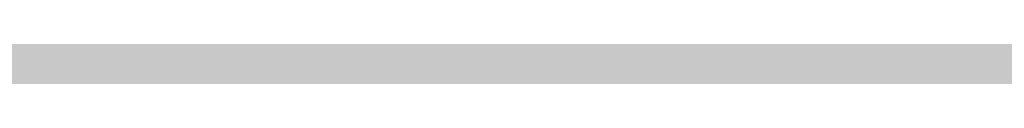
# Model space of a CAD drawing. Units: millimetres. Extents: x 0 to 2267, y 0 to 1823.
# Tile 105 of 256: x 1600.369 to 1605.705, y 1232.061 to 1232.196. Entities that reach past the tile are written whole.
import ezdxf

# ---------------------------------------------------------------- set-up
doc = ezdxf.new("R2010")
doc.units = ezdxf.units.MM
doc.header["$MEASUREMENT"] = 0
doc.layers.add('M-DIMS', color=2, linetype='Continuous', lineweight=25)
doc.layers.add('M-HATC', color=252, linetype='Continuous', lineweight=18)
doc.styles.get("Standard").update_dxf_attribs({"font": 'arial.ttf'})
doc.dimstyles.get("Standard").update_dxf_attribs({"dimtxt": 7, "dimasz": 4, "dimexe": 0.18, "dimexo": 0.0625, "dimgap": 0.09, "dimtad": 0, "dimdec": 0, "dimzin": 0, "dimdsep": 46, "dimtxsty": 'Standard', "dimcen": 0.09, "dimadec": 0, "dimazin": 0, "dimtfac": 1, "dimtdec": 0, "dimtofl": 0, "dimtmove": 0, "dimatfit": 3, "dimfxl": 1, "dimtolj": 1, "dimtzin": 0, "dimarcsym": 0})

# ---------------------------------------------------------------- blocks, each defined once
blk = doc.blocks.new('*D19')
at = {"layer": 'Defpoints', "color": 0, "transparency": 16777216}
for p in [(1605.3399, 1483.3044), (1445.5291, 1333.8851)]:
    blk.add_point(p, dxfattribs=at)
at = {"layer": 'M-DIMS', "color": 0, "lineweight": -2, "transparency": 16777216}
for p, q in [((1605.3399, 1483.2144), (1605.3399, 1483.3944)), ((1605.2499, 1483.3044), (1605.4299, 1483.3044)), ((1366.3244, 1259.8306), (1442.6072, 1331.1532))]:
    blk.add_line(p, q, dxfattribs=at)
at = {"layer": 'M-DIMS', "color": 0, "transparency": 16777216}
blk.add_solid([(1442.1519, 1331.6402), (1443.0625, 1330.6663), (1445.5291, 1333.8851)], dxfattribs=at)
at = {"layer": 'M-DIMS', "color": 0, "transparency": 16777216, "insert": (1349.6425, 1244.2335), "char_height": 7, "attachment_point": 5, "rotation": 43.0753}
blk.add_mtext('\\A1;2X R218.8', dxfattribs=at)

msp = doc.modelspace()

# ---------------------------------------------------------------- hatches: boundary and pattern name
at = {"layer": 'M-HATC'}
h = msp.add_hatch(color=256, dxfattribs=at)
h.dxf.hatch_style = 1
h.paths.add_polyline_path([(2055.771, 1603.062), (1381.0868, 1603.062), (1381.0868, 1598.062), (2055.771, 1598.062)])
h.paths.add_polyline_path([(2055.771, 1598.062), (1381.0868, 1598.062), (1381.0868, 1593.062), (2055.771, 1593.062)])
h.paths.add_polyline_path([(2051.3074, 1536.7609), (1385.5504, 1536.7609), (1385.5504, 1526.7609), (1387.5504, 1526.7609), (1388.5366, 1525.0528), (1385.3319, 1521.2335), (1385.3319, 1521.2226), (2050.2542, 1522.7491), (2048.3212, 1525.0528), (2049.3074, 1526.7609), (2051.3074, 1526.7609)])
edge = h.paths.add_edge_path()
edge.add_arc((1847.5345, 1379.1492), 135, 222.603061, 222.890851, ccw=False)
edge.add_line((1748.1663, 1287.7656), (1683.0921, 1287.7656))
edge.add_arc((1583.7239, 1379.1492), 135, 317.109149, 317.396939, ccw=False)
edge.add_arc((1678.9686, 1290.6707), 5, 222.8909, 317.1091, ccw=False)
edge.add_arc((1774.2133, 1379.1492), 135, 222.603061, 222.890851, ccw=False)
edge.add_line((1674.8451, 1287.7656), (1609.7709, 1287.7656))
edge.add_arc((1510.4027, 1379.1492), 135, 317.109149, 317.396939, ccw=False)
edge.add_arc((1605.6474, 1290.6707), 5, 222.8909, 317.1091, ccw=False)
edge.add_arc((1700.8921, 1379.1492), 135, 222.603061, 222.890851, ccw=False)
edge.add_line((1601.5239, 1287.7656), (1536.4497, 1287.7656))
edge.add_arc((1437.0815, 1379.1492), 135, 317.109149, 317.396939, ccw=False)
edge.add_arc((1532.3262, 1290.6707), 5, 222.8909, 317.1091, ccw=False)
edge.add_arc((1627.5709, 1379.1492), 135, 222.603061, 222.890851, ccw=False)
edge.add_line((1528.2027, 1287.7656), (1505.9289, 1287.7656))
edge.add_spline(control_points=[(1505.9289, 1287.7656), (1504.2622, 1287.7656), (1504.2622, 1282.7656), (1505.9289, 1282.7656)], knot_values=[0, 0, 0, 0, 5, 5, 5, 5], degree=3, periodic=0)
edge.add_line((1505.9289, 1282.7656), (1930.9289, 1282.7656))
edge.add_spline(control_points=[(1930.9289, 1282.7656), (1932.5956, 1282.7656), (1932.5956, 1287.7656), (1930.9289, 1287.7656)], knot_values=[0, 0, 0, 0, 5, 5, 5, 5], degree=3, periodic=0)
edge.add_line((1930.9289, 1287.7656), (1903.0557, 1287.7656))
edge.add_arc((1803.6875, 1379.1492), 135, 317.109149, 317.396939, ccw=False)
edge.add_arc((1898.9322, 1290.6707), 5, 222.8909, 317.1091, ccw=False)
edge.add_arc((1994.1769, 1379.1492), 135, 222.603061, 222.890851, ccw=False)
edge.add_line((1894.8087, 1287.7656), (1829.7345, 1287.7656))
edge.add_arc((1730.3663, 1379.1492), 135, 317.109149, 317.396939, ccw=False)
edge.add_arc((1825.611, 1290.6707), 5, 222.8909, 317.1091, ccw=False)
edge.add_arc((1920.8557, 1379.1492), 135, 222.603061, 222.890851, ccw=False)
edge.add_line((1821.4875, 1287.7656), (1756.4133, 1287.7656))
edge.add_arc((1657.0451, 1379.1492), 135, 317.109149, 317.396939, ccw=False)
edge.add_arc((1752.2898, 1290.6707), 5, 222.8909, 317.1091, ccw=False)
edge = h.paths.add_edge_path()
edge.add_spline(control_points=[(1843.4289, 1227.2475), (1845.0956, 1227.2475), (1845.0956, 1232.2475), (1843.4289, 1232.2475)], knot_values=[0, 0, 0, 0, 5, 5, 5, 5], degree=3, periodic=0)
edge.add_line((1843.4289, 1232.2475), (1593.4289, 1232.2475))
edge.add_spline(control_points=[(1593.4289, 1232.2475), (1591.7622, 1232.2475), (1591.7622, 1227.2475), (1593.4289, 1227.2475)], knot_values=[0, 0, 0, 0, 5, 5, 5, 5], degree=3, periodic=0)
edge.add_line((1593.4289, 1227.2475), (1843.4289, 1227.2475))
h.paths.add_polyline_path([(1905.9289, 1127.4171), (1530.9289, 1127.4171, 0.414214), (1520.9289, 1117.4171), (1530.9289, 1117.4171), (1915.9289, 1117.4171, 0.414214)])
edge = h.paths.add_edge_path()
edge.add_arc((1397.0858, 1498.4078), 12.7299, 90.78215, 190.87871, ccw=False)
edge.add_line((1396.912, 1511.1365), (1428.0097, 1511.3488))
edge.add_line((1428.0097, 1511.3488), (1433.0097, 1511.3488))
edge.add_line((1433.0097, 1511.3488), (1434.439, 1511.3488))
edge.add_arc((1419.474, 1498.0804), 20, 41.561, 74.08211)
edge.add_line((1424.9592, 1517.3135), (1399.9351, 1517.2561))
edge.add_spline(control_points=[(1399.9307, 1517.2561), (1399.884, 1517.2131), (1399.8328, 1517.1689), (1399.7774, 1517.1236)], knot_values=[11.567499, 11.567499, 11.567499, 11.567499, 11.814249, 11.814249, 11.814249, 11.814249], degree=3, periodic=0)
edge.add_spline(control_points=[(1399.6328, 1517.0099), (1399.5831, 1516.9721), (1399.5307, 1516.9338), (1399.4759, 1516.8947)], knot_values=[11.167718, 11.167718, 11.167718, 11.167718, 11.365188, 11.365188, 11.365188, 11.365188], degree=3, periodic=0)
edge.add_spline(control_points=[(1399.3398, 1516.8001), (1399.1514, 1516.6719), (1398.9384, 1516.5377), (1398.704, 1516.3994)], knot_values=[10.376405, 10.376405, 10.376405, 10.376405, 11.00994, 11.00994, 11.00994, 11.00994], degree=3, periodic=0)
edge.add_spline(control_points=[(1398.6572, 1516.3719), (1398.5789, 1516.326), (1398.4983, 1516.2797), (1398.4155, 1516.2331)], knot_values=[10.125175, 10.125175, 10.125175, 10.125175, 10.334406, 10.334406, 10.334406, 10.334406], degree=3, periodic=0)
edge.add_spline(control_points=[(1398.2642, 1516.1487), (1398.196, 1516.1111), (1398.1263, 1516.0732), (1398.0555, 1516.0351)], knot_values=[9.832246, 9.832246, 9.832246, 9.832246, 9.999658, 9.999658, 9.999658, 9.999658], degree=3, periodic=0)
edge.add_spline(control_points=[(1397.9987, 1516.0048), (1397.7312, 1515.8621), (1397.446, 1515.7171), (1397.1466, 1515.5714)], knot_values=[9.161808, 9.161808, 9.161808, 9.161808, 9.787769, 9.787769, 9.787769, 9.787769], degree=3, periodic=0)
edge.add_spline(control_points=[(1397.1466, 1515.5714), (1396.8418, 1515.423), (1396.5222, 1515.274), (1396.1914, 1515.1262)], knot_values=[8.524455, 8.524455, 8.524455, 8.524455, 9.161808, 9.161808, 9.161808, 9.161808], degree=3, periodic=0)
edge.add_spline(control_points=[(1396.0777, 1515.0756), (1395.9854, 1515.0348), (1395.8922, 1514.994), (1395.7983, 1514.9534)], knot_values=[8.275193, 8.275193, 8.275193, 8.275193, 8.451726, 8.451726, 8.451726, 8.451726], degree=3, periodic=0)
edge.add_spline(control_points=[(1395.6018, 1514.8691), (1395.4997, 1514.8257), (1395.3968, 1514.7824), (1395.2932, 1514.7394)], knot_values=[7.962917, 7.962917, 7.962917, 7.962917, 8.152764, 8.152764, 8.152764, 8.152764], degree=3, periodic=0)
edge.add_spline(control_points=[(1395.2116, 1514.7057), (1394.8278, 1514.5475), (1394.4345, 1514.3929), (1394.0364, 1514.2442)], knot_values=[7.21254, 7.21254, 7.21254, 7.21254, 7.913148, 7.913148, 7.913148, 7.913148], degree=3, periodic=0)
edge.add_spline(control_points=[(1394.0364, 1514.2442), (1393.7076, 1514.1214), (1393.3754, 1514.0027), (1393.0427, 1513.8895)], knot_values=[6.633733, 6.633733, 6.633733, 6.633733, 7.21254, 7.21254, 7.21254, 7.21254], degree=3, periodic=0)
edge.add_spline(control_points=[(1392.8214, 1513.815), (1392.7198, 1513.7812), (1392.6181, 1513.7479), (1392.5166, 1513.7152)], knot_values=[6.328796, 6.328796, 6.328796, 6.328796, 6.505493, 6.505493, 6.505493, 6.505493], degree=3, periodic=0)
edge.add_spline(control_points=[(1392.5166, 1513.7152), (1392.3187, 1513.6515), (1392.1212, 1513.59), (1391.9244, 1513.531)], knot_values=[5.984605, 5.984605, 5.984605, 5.984605, 6.328796, 6.328796, 6.328796, 6.328796], degree=3, periodic=0)
edge.add_spline(control_points=[(1391.7915, 1513.4915), (1391.3122, 1513.3501), (1390.8384, 1513.2239), (1390.3784, 1513.1171)], knot_values=[5.066697, 5.066697, 5.066697, 5.066697, 5.907055, 5.907055, 5.907055, 5.907055], degree=3, periodic=0)
edge.add_spline(control_points=[(1390.3784, 1513.1171), (1390.1797, 1513.071), (1389.9836, 1513.0284), (1389.7907, 1512.9899)], knot_values=[4.70367, 4.70367, 4.70367, 4.70367, 5.066695, 5.066695, 5.066695, 5.066695], degree=3, periodic=0)
edge.add_spline(control_points=[(1389.422, 1512.9204), (1389.2459, 1512.8892), (1389.0729, 1512.8617), (1388.9036, 1512.8381)], knot_values=[4.130571, 4.130571, 4.130571, 4.130571, 4.469816, 4.469816, 4.469816, 4.469816], degree=3, periodic=0)
edge.add_spline(control_points=[(1388.9036, 1512.8381), (1388.591, 1512.7946), (1388.2911, 1512.7644), (1388.0071, 1512.7494)], knot_values=[3.504031, 3.504031, 3.504031, 3.504031, 4.130571, 4.130571, 4.130571, 4.130571], degree=3, periodic=0)
edge.add_spline(control_points=[(1387.9356, 1512.7459), (1387.8538, 1512.7423), (1387.7733, 1512.74), (1387.6944, 1512.739)], knot_values=[3.268866, 3.268866, 3.268866, 3.268866, 3.451164, 3.451164, 3.451164, 3.451164], degree=3, periodic=0)
edge.add_spline(control_points=[(1387.3351, 1512.7443), (1387.2076, 1512.7499), (1387.0847, 1512.7597), (1386.967, 1512.7739)], knot_values=[2.670686, 2.670686, 2.670686, 2.670686, 2.984, 2.984, 2.984, 2.984], degree=3, periodic=0)
edge.add_spline(control_points=[(1386.8327, 1512.7922), (1386.8209, 1512.7941), (1386.8092, 1512.7959), (1386.7975, 1512.7979)], knot_values=[2.516981, 2.516981, 2.516981, 2.516981, 2.549528, 2.549528, 2.549528, 2.549528], degree=3, periodic=0)
edge.add_spline(control_points=[(1386.4526, 1512.8735), (1386.4257, 1512.881), (1386.3993, 1512.889), (1386.3733, 1512.8972)], knot_values=[2.095869, 2.095869, 2.095869, 2.095869, 2.17941, 2.17941, 2.17941, 2.17941], degree=3, periodic=0)
edge.add_spline(control_points=[(1386.0691, 1513.0189), (1386.0634, 1513.0217), (1386.0577, 1513.0246), (1386.052, 1513.0275)], knot_values=[1.72453, 1.72453, 1.72453, 1.72453, 1.745933, 1.745933, 1.745933, 1.745933], degree=3, periodic=0)
edge.add_arc((1399.474, 1498.0804), 20, 131.82432, 180)
edge.add_arc((1630.3336, 1505.5484), 250.9708, 181.705176, 236.427975)
edge.add_arc((1605.3399, 1483.3044), 218.7822, 238.660829, 243.34961)
edge.add_arc((1647.0911, 1510.3592), 262.8986, 183.129836, 237.853442, ccw=False)
h.paths.add_polyline_path([(1406.5369, 1391.9644, 0.149382), (1491.5506, 1296.4418, -0.129517)], flags=17)
edge = h.paths.add_edge_path()
edge.add_arc((2037.3838, 1498.0804), 20, 0, 48.26587)
edge.add_spline(control_points=[(2050.6973, 1513.0052), (2050.6512, 1512.9847), (2050.6034, 1512.9655), (2050.5539, 1512.9477)], knot_values=[1.835652, 1.835652, 1.835652, 1.835652, 2.000781, 2.000781, 2.000781, 2.000781], degree=3, periodic=0)
edge.add_spline(control_points=[(2050.4616, 1512.9166), (2050.479, 1512.9221), (2050.4963, 1512.9277), (2050.5133, 1512.9335)], knot_values=[2.045477, 2.045477, 2.045477, 2.045477, 2.101389, 2.101389, 2.101389, 2.101389], degree=3, periodic=0)
edge.add_spline(control_points=[(2050.129, 1512.8342), (2050.1984, 1512.8473), (2050.2657, 1512.8623), (2050.3308, 1512.8792)], knot_values=[2.237629, 2.237629, 2.237629, 2.237629, 2.435841, 2.435841, 2.435841, 2.435841], degree=3, periodic=0)
edge.add_spline(control_points=[(2050.0946, 1512.8278), (2050.1061, 1512.8299), (2050.1176, 1512.832), (2050.129, 1512.8342)], knot_values=[2.435841, 2.435841, 2.435841, 2.435841, 2.468321, 2.468321, 2.468321, 2.468321], degree=3, periodic=0)
edge.add_spline(control_points=[(2049.7843, 1512.7851), (2049.8552, 1512.7922), (2049.9243, 1512.8008), (2049.9917, 1512.8109)], knot_values=[2.563852, 2.563852, 2.563852, 2.563852, 2.748541, 2.748541, 2.748541, 2.748541], degree=3, periodic=0)
edge.add_spline(control_points=[(2049.4052, 1512.7617), (2049.5364, 1512.7653), (2049.6629, 1512.773), (2049.7843, 1512.7851)], knot_values=[2.748541, 2.748541, 2.748541, 2.748541, 3.064882, 3.064882, 3.064882, 3.064882], degree=3, periodic=0)
edge.add_spline(control_points=[(2049.1698, 1512.7597), (2049.2336, 1512.7591), (2049.2965, 1512.7594), (2049.3584, 1512.7606)], knot_values=[3.102309, 3.102309, 3.102309, 3.102309, 3.2503, 3.2503, 3.2503, 3.2503], degree=3, periodic=0)
edge.add_spline(control_points=[(2048.8573, 1512.7691), (2048.9638, 1512.7638), (2049.068, 1512.7606), (2049.1698, 1512.7597)], knot_values=[3.2503, 3.2503, 3.2503, 3.2503, 3.486069, 3.486069, 3.486069, 3.486069], degree=3, periodic=0)
edge.add_spline(control_points=[(2048.6924, 1512.7789), (2048.3729, 1512.8009), (2048.0345, 1512.8411), (2047.6817, 1512.897)], knot_values=[3.606429, 3.606429, 3.606429, 3.606429, 4.2989, 4.2989, 4.2989, 4.2989], degree=3, periodic=0)
edge.add_spline(control_points=[(2047.6817, 1512.897), (2047.5458, 1512.9185), (2047.4077, 1512.9424), (2047.2678, 1512.9685)], knot_values=[4.2989, 4.2989, 4.2989, 4.2989, 4.565769, 4.565769, 4.565769, 4.565769], degree=3, periodic=0)
edge.add_spline(control_points=[(2047.2678, 1512.9685), (2047.1449, 1512.9914), (2047.0207, 1513.016), (2046.8951, 1513.0422)], knot_values=[4.565769, 4.565769, 4.565769, 4.565769, 4.799971, 4.799971, 4.799971, 4.799971], degree=3, periodic=0)
edge.add_spline(control_points=[(2046.8951, 1513.0422), (2046.5286, 1513.1188), (2046.1513, 1513.209), (2045.7676, 1513.3107)], knot_values=[4.799971, 4.799971, 4.799971, 4.799971, 5.483718, 5.483718, 5.483718, 5.483718], degree=3, periodic=0)
edge.add_spline(control_points=[(2045.7676, 1513.3107), (2045.3724, 1513.4154), (2044.9704, 1513.5322), (2044.5662, 1513.6588)], knot_values=[5.483718, 5.483718, 5.483718, 5.483718, 6.187866, 6.187866, 6.187866, 6.187866], degree=3, periodic=0)
edge.add_spline(control_points=[(2044.5662, 1513.6588), (2044.4149, 1513.7061), (2044.2633, 1513.7549), (2044.1116, 1513.8048)], knot_values=[6.187866, 6.187866, 6.187866, 6.187866, 6.451551, 6.451551, 6.451551, 6.451551], degree=3, periodic=0)
edge.add_spline(control_points=[(2044.1116, 1513.8048), (2043.9967, 1513.8427), (2043.8817, 1513.8813), (2043.7668, 1513.9205)], knot_values=[6.451551, 6.451551, 6.451551, 6.451551, 6.651434, 6.651434, 6.651434, 6.651434], degree=3, periodic=0)
edge.add_spline(control_points=[(2043.7668, 1513.9205), (2043.3716, 1514.0554), (2042.9774, 1514.1979), (2042.5886, 1514.3458)], knot_values=[6.651434, 6.651434, 6.651434, 6.651434, 7.338879, 7.338879, 7.338879, 7.338879], degree=3, periodic=0)
edge.add_spline(control_points=[(2042.5886, 1514.3458), (2042.1643, 1514.5071), (2041.7465, 1514.6749), (2041.3409, 1514.846)], knot_values=[7.338879, 7.338879, 7.338879, 7.338879, 8.089209, 8.089209, 8.089209, 8.089209], degree=3, periodic=0)
edge.add_spline(control_points=[(2041.3409, 1514.846), (2041.1028, 1514.9465), (2040.869, 1515.0481), (2040.6405, 1515.1502)], knot_values=[8.089209, 8.089209, 8.089209, 8.089209, 8.529587, 8.529587, 8.529587, 8.529587], degree=3, periodic=0)
edge.add_spline(control_points=[(2040.51, 1515.2089), (2040.0824, 1515.4022), (2039.6747, 1515.5971), (2039.295, 1515.7894)], knot_values=[8.613818, 8.613818, 8.613818, 8.613818, 9.44571, 9.44571, 9.44571, 9.44571], degree=3, periodic=0)
edge.add_spline(control_points=[(2039.295, 1515.7894), (2039.0618, 1515.9075), (2038.8391, 1516.0246), (2038.6288, 1516.1398)], knot_values=[9.44571, 9.44571, 9.44571, 9.44571, 9.956404, 9.956404, 9.956404, 9.956404], degree=3, periodic=0)
edge.add_spline(control_points=[(2038.6288, 1516.1398), (2038.5187, 1516.2001), (2038.4121, 1516.2598), (2038.309, 1516.3189)], knot_values=[9.956404, 9.956404, 9.956404, 9.956404, 10.223542, 10.223542, 10.223542, 10.223542], degree=3, periodic=0)
edge.add_spline(control_points=[(2038.309, 1516.3189), (2038.2138, 1516.3735), (2038.1216, 1516.4276), (2038.0328, 1516.481)], knot_values=[10.223542, 10.223542, 10.223542, 10.223542, 10.47051, 10.47051, 10.47051, 10.47051], degree=3, periodic=0)
edge.add_spline(control_points=[(2038.0328, 1516.481), (2037.7855, 1516.6296), (2037.5639, 1516.773), (2037.3722, 1516.909)], knot_values=[10.47051, 10.47051, 10.47051, 10.47051, 11.15767, 11.15767, 11.15767, 11.15767], degree=3, periodic=0)
edge.add_spline(control_points=[(2037.3722, 1516.909), (2037.2789, 1516.9752), (2037.1927, 1517.0396), (2037.1142, 1517.102)], knot_values=[11.15767, 11.15767, 11.15767, 11.15767, 11.49227, 11.49227, 11.49227, 11.49227], degree=3, periodic=0)
edge.add_spline(control_points=[(2036.8564, 1517.3259), (2036.9148, 1517.2692), (2036.9814, 1517.2103), (2037.0557, 1517.1492)], knot_values=[11.577341, 11.577341, 11.577341, 11.577341, 11.91035, 11.91035, 11.91035, 11.91035], degree=3, periodic=0)
edge.add_spline(control_points=[(2036.8074, 1517.3748), (2036.823, 1517.3587), (2036.8393, 1517.3424), (2036.8564, 1517.3259)], knot_values=[11.91035, 11.91035, 11.91035, 11.91035, 12.007402, 12.007402, 12.007402, 12.007402], degree=3, periodic=0)
edge.add_spline(control_points=[(2036.7017, 1517.494), (2036.7104, 1517.483), (2036.7196, 1517.4719), (2036.7291, 1517.4606)], knot_values=[12.184155, 12.184155, 12.184155, 12.184155, 12.255409, 12.255409, 12.255409, 12.255409], degree=3, periodic=0)
edge.add_spline(control_points=[(2036.6159, 1517.6205), (2036.62, 1517.613), (2036.6243, 1517.6055), (2036.6289, 1517.5979)], knot_values=[12.487913, 12.487913, 12.487913, 12.487913, 12.541035, 12.541035, 12.541035, 12.541035], degree=3, periodic=0)
edge.add_spline(control_points=[(2036.5635, 1517.786), (2036.5637, 1517.7794), (2036.5642, 1517.7726), (2036.565, 1517.7658)], knot_values=[12.911761, 12.911761, 12.911761, 12.911761, 12.968286, 12.968286, 12.968286, 12.968286], degree=3, periodic=0)
edge.add_spline(control_points=[(2036.6166, 1517.9304), (2036.6125, 1517.9259), (2036.6086, 1517.9212), (2036.6049, 1517.9165)], knot_values=[13.382527, 13.382527, 13.382527, 13.382527, 13.433791, 13.433791, 13.433791, 13.433791], degree=3, periodic=0)
edge.add_spline(control_points=[(2036.749, 1518.017), (2036.7361, 1518.0116), (2036.7239, 1518.006), (2036.7124, 1518.0002)], knot_values=[13.726299, 13.726299, 13.726299, 13.726299, 13.809928, 13.809928, 13.809928, 13.809928], degree=3, periodic=0)
edge.add_spline(control_points=[(2036.8604, 1518.0528), (2036.8386, 1518.0474), (2036.8181, 1518.0416), (2036.7988, 1518.0353)], knot_values=[13.910887, 13.910887, 13.910887, 13.910887, 14.02153, 14.02153, 14.02153, 14.02153], degree=3, periodic=0)
edge.add_line((2036.9639, 1518.0804), (2032.3838, 1518.0804))
edge.add_line((2032.3838, 1518.0804), (2027.3838, 1518.0804))
edge.add_line((2027.3838, 1518.0804), (2022.3838, 1518.0804))
edge.add_line((2022.3838, 1518.0804), (2017.3838, 1518.0804))
edge.add_arc((2017.3838, 1498.0804), 20, 90, 138.439)
edge.add_line((2002.4188, 1511.3488), (2003.8481, 1511.3488))
edge.add_line((2003.8481, 1511.3488), (2008.8481, 1511.3488))
edge.add_line((2008.8481, 1511.3488), (2039.772, 1511.1377))
edge.add_arc((2039.772, 1498.4078), 12.7299, -10.87871, 90, ccw=False)
edge.add_arc((1789.7668, 1510.3592), 262.8986, 302.146558, 356.870164, ccw=False)
edge.add_arc((1831.5179, 1483.3044), 218.7822, 296.65039, 301.339171)
edge.add_arc((1806.5242, 1505.5484), 250.9708, 303.572025, 358.294824)
h.paths.add_polyline_path([(2030.321, 1391.9644, -0.129517), (1945.3072, 1296.4418, 0.149382)], flags=17)
edge = h.paths.add_edge_path()
edge.add_spline(control_points=[(2037.2464, 1518.0821), (2037.2898, 1518.081), (2037.3355, 1518.0804), (2037.3838, 1518.0804)], knot_values=[0.000012, 0.000012, 0.000012, 0.000012, 0.144754, 0.144754, 0.144754, 0.144754], degree=3, periodic=0)
edge.add_line((2037.3357, 1518.0804), (2037.0096, 1518.0804))
edge.add_spline(control_points=[(2037.0096, 1518.0804), (2036.9822, 1518.0768), (2036.956, 1518.0727), (2036.9312, 1518.0681)], knot_values=[14.13465, 14.13465, 14.13465, 14.13465, 14.247197, 14.247197, 14.247197, 14.247197], degree=3, periodic=0)
edge.add_spline(control_points=[(2036.9312, 1518.0681), (2036.9276, 1518.0674), (2036.9241, 1518.0667), (2036.9205, 1518.0661)], knot_values=[14.118315, 14.118315, 14.118315, 14.118315, 14.13465, 14.13465, 14.13465, 14.13465], degree=3, periodic=0)
edge.add_spline(control_points=[(2036.9205, 1518.0661), (2036.9118, 1518.0644), (2036.9032, 1518.0626), (2036.8948, 1518.0608)], knot_values=[14.078086, 14.078086, 14.078086, 14.078086, 14.118315, 14.118315, 14.118315, 14.118315], degree=3, periodic=0)
edge.add_spline(control_points=[(2036.8948, 1518.0608), (2036.883, 1518.0583), (2036.8716, 1518.0556), (2036.8604, 1518.0528)], knot_values=[14.02153, 14.02153, 14.02153, 14.02153, 14.078086, 14.078086, 14.078086, 14.078086], degree=3, periodic=0)
edge.add_spline(control_points=[(2036.8604, 1518.0528), (2036.8386, 1518.0474), (2036.8181, 1518.0416), (2036.7988, 1518.0353)], knot_values=[13.910887, 13.910887, 13.910887, 13.910887, 14.02153, 14.02153, 14.02153, 14.02153], degree=3, periodic=0)
edge.add_spline(control_points=[(2036.7988, 1518.0353), (2036.7981, 1518.035), (2036.7974, 1518.0348), (2036.7967, 1518.0346)], knot_values=[13.906906, 13.906906, 13.906906, 13.906906, 13.910887, 13.910887, 13.910887, 13.910887], degree=3, periodic=0)
edge.add_spline(control_points=[(2036.7967, 1518.0346), (2036.7882, 1518.0318), (2036.7799, 1518.0289), (2036.7719, 1518.0259)], knot_values=[13.857826, 13.857826, 13.857826, 13.857826, 13.906906, 13.906906, 13.906906, 13.906906], degree=3, periodic=0)
edge.add_spline(control_points=[(2036.7719, 1518.0259), (2036.764, 1518.023), (2036.7564, 1518.02), (2036.749, 1518.017)], knot_values=[13.809928, 13.809928, 13.809928, 13.809928, 13.857826, 13.857826, 13.857826, 13.857826], degree=3, periodic=0)
edge.add_spline(control_points=[(2036.749, 1518.017), (2036.7361, 1518.0116), (2036.7239, 1518.006), (2036.7124, 1518.0002)], knot_values=[13.726299, 13.726299, 13.726299, 13.726299, 13.809928, 13.809928, 13.809928, 13.809928], degree=3, periodic=0)
edge.add_spline(control_points=[(2036.7124, 1518.0002), (2036.7121, 1518), (2036.7118, 1517.9999), (2036.7115, 1517.9997)], knot_values=[13.723993, 13.723993, 13.723993, 13.723993, 13.726299, 13.726299, 13.726299, 13.726299], degree=3, periodic=0)
edge.add_spline(control_points=[(2036.7115, 1517.9997), (2036.7063, 1517.9971), (2036.7013, 1517.9944), (2036.6965, 1517.9917)], knot_values=[13.686536, 13.686536, 13.686536, 13.686536, 13.723993, 13.723993, 13.723993, 13.723993], degree=3, periodic=0)
edge.add_spline(control_points=[(2036.6965, 1517.9917), (2036.6919, 1517.9891), (2036.6874, 1517.9865), (2036.6831, 1517.9839)], knot_values=[13.651251, 13.651251, 13.651251, 13.651251, 13.686536, 13.686536, 13.686536, 13.686536], degree=3, periodic=0)
edge.add_spline(control_points=[(2036.6831, 1517.9839), (2036.6764, 1517.9798), (2036.67, 1517.9757), (2036.6639, 1517.9714)], knot_values=[13.596804, 13.596804, 13.596804, 13.596804, 13.651251, 13.651251, 13.651251, 13.651251], degree=3, periodic=0)
edge.add_spline(control_points=[(2036.6639, 1517.9714), (2036.6636, 1517.9712), (2036.6633, 1517.9709), (2036.6629, 1517.9707)], knot_values=[13.593956, 13.593956, 13.593956, 13.593956, 13.596804, 13.596804, 13.596804, 13.596804], degree=3, periodic=0)
edge.add_spline(control_points=[(2036.6629, 1517.9707), (2036.6603, 1517.9689), (2036.6577, 1517.967), (2036.6552, 1517.9651)], knot_values=[13.570322, 13.570322, 13.570322, 13.570322, 13.593956, 13.593956, 13.593956, 13.593956], degree=3, periodic=0)
edge.add_spline(control_points=[(2036.6552, 1517.9651), (2036.6525, 1517.9631), (2036.6499, 1517.9611), (2036.6474, 1517.9591)], knot_values=[13.545477, 13.545477, 13.545477, 13.545477, 13.570322, 13.570322, 13.570322, 13.570322], degree=3, periodic=0)
edge.add_spline(control_points=[(2036.6474, 1517.9591), (2036.6472, 1517.9589), (2036.6471, 1517.9588), (2036.6469, 1517.9587)], knot_values=[13.543931, 13.543931, 13.543931, 13.543931, 13.545477, 13.545477, 13.545477, 13.545477], degree=3, periodic=0)
edge.add_spline(control_points=[(2036.6469, 1517.9587), (2036.6412, 1517.9541), (2036.6358, 1517.9494), (2036.6307, 1517.9447)], knot_values=[13.488237, 13.488237, 13.488237, 13.488237, 13.543931, 13.543931, 13.543931, 13.543931], degree=3, periodic=0)
edge.add_spline(control_points=[(2036.6307, 1517.9447), (2036.6282, 1517.9423), (2036.6257, 1517.9399), (2036.6233, 1517.9374)], knot_values=[13.460307, 13.460307, 13.460307, 13.460307, 13.488237, 13.488237, 13.488237, 13.488237], degree=3, periodic=0)
edge.add_spline(control_points=[(2036.6233, 1517.9374), (2036.6215, 1517.9356), (2036.6198, 1517.9338), (2036.6181, 1517.932)], knot_values=[13.439712, 13.439712, 13.439712, 13.439712, 13.460307, 13.460307, 13.460307, 13.460307], degree=3, periodic=0)
edge.add_spline(control_points=[(2036.6181, 1517.932), (2036.6176, 1517.9315), (2036.6171, 1517.9309), (2036.6166, 1517.9304)], knot_values=[13.433791, 13.433791, 13.433791, 13.433791, 13.439712, 13.439712, 13.439712, 13.439712], degree=3, periodic=0)
edge.add_spline(control_points=[(2036.6166, 1517.9304), (2036.6125, 1517.9259), (2036.6086, 1517.9212), (2036.6049, 1517.9165)], knot_values=[13.382527, 13.382527, 13.382527, 13.382527, 13.433791, 13.433791, 13.433791, 13.433791], degree=3, periodic=0)
edge.add_spline(control_points=[(2036.6049, 1517.9165), (2036.6026, 1517.9135), (2036.6004, 1517.9104), (2036.5982, 1517.9074)], knot_values=[13.350017, 13.350017, 13.350017, 13.350017, 13.382527, 13.382527, 13.382527, 13.382527], degree=3, periodic=0)
edge.add_spline(control_points=[(2036.5982, 1517.9074), (2036.5972, 1517.9059), (2036.5962, 1517.9043), (2036.5952, 1517.9028)], knot_values=[13.333922, 13.333922, 13.333922, 13.333922, 13.350017, 13.350017, 13.350017, 13.350017], degree=3, periodic=0)
edge.add_spline(control_points=[(2036.5952, 1517.9028), (2036.5945, 1517.9018), (2036.5939, 1517.9009), (2036.5933, 1517.8999)], knot_values=[13.323828, 13.323828, 13.323828, 13.323828, 13.333922, 13.333922, 13.333922, 13.333922], degree=3, periodic=0)
edge.add_spline(control_points=[(2036.5933, 1517.8999), (2036.5905, 1517.8955), (2036.5879, 1517.8909), (2036.5855, 1517.8864)], knot_values=[13.277545, 13.277545, 13.277545, 13.277545, 13.323828, 13.323828, 13.323828, 13.323828], degree=3, periodic=0)
edge.add_spline(control_points=[(2036.5855, 1517.8864), (2036.5836, 1517.8827), (2036.5817, 1517.8789), (2036.5801, 1517.8751)], knot_values=[13.240119, 13.240119, 13.240119, 13.240119, 13.277545, 13.277545, 13.277545, 13.277545], degree=3, periodic=0)
edge.add_spline(control_points=[(2036.5801, 1517.8751), (2036.5795, 1517.8739), (2036.579, 1517.8727), (2036.5785, 1517.8715)], knot_values=[13.228211, 13.228211, 13.228211, 13.228211, 13.240119, 13.240119, 13.240119, 13.240119], degree=3, periodic=0)
edge.add_spline(control_points=[(2036.5785, 1517.8715), (2036.578, 1517.8702), (2036.5774, 1517.869), (2036.5769, 1517.8677)], knot_values=[13.215717, 13.215717, 13.215717, 13.215717, 13.228211, 13.228211, 13.228211, 13.228211], degree=3, periodic=0)
edge.add_spline(control_points=[(2036.5769, 1517.8677), (2036.5755, 1517.864), (2036.5741, 1517.8603), (2036.5729, 1517.8565)], knot_values=[13.179847, 13.179847, 13.179847, 13.179847, 13.215717, 13.215717, 13.215717, 13.215717], degree=3, periodic=0)
edge.add_spline(control_points=[(2036.5729, 1517.8565), (2036.5713, 1517.8515), (2036.5699, 1517.8464), (2036.5687, 1517.8413)], knot_values=[13.132017, 13.132017, 13.132017, 13.132017, 13.179847, 13.179847, 13.179847, 13.179847], degree=3, periodic=0)
edge.add_spline(control_points=[(2036.5687, 1517.8413), (2036.5684, 1517.8402), (2036.5682, 1517.8392), (2036.568, 1517.8382)], knot_values=[13.122482, 13.122482, 13.122482, 13.122482, 13.132017, 13.132017, 13.132017, 13.132017], degree=3, periodic=0)
edge.add_spline(control_points=[(2036.568, 1517.8382), (2036.5676, 1517.8363), (2036.5672, 1517.8345), (2036.5669, 1517.8327)], knot_values=[13.105592, 13.105592, 13.105592, 13.105592, 13.122482, 13.122482, 13.122482, 13.122482], degree=3, periodic=0)
edge.add_spline(control_points=[(2036.5669, 1517.8327), (2036.5662, 1517.8292), (2036.5657, 1517.8257), (2036.5652, 1517.8222)], knot_values=[13.074063, 13.074063, 13.074063, 13.074063, 13.105592, 13.105592, 13.105592, 13.105592], degree=3, periodic=0)
edge.add_spline(control_points=[(2036.5652, 1517.8222), (2036.5652, 1517.8222), (2036.5652, 1517.8222), (2036.5652, 1517.8222)], knot_values=[13.074043, 13.074043, 13.074043, 13.074043, 13.074063, 13.074063, 13.074063, 13.074063], degree=3, periodic=0)
edge.add_spline(control_points=[(2036.5652, 1517.8222), (2036.5644, 1517.8164), (2036.5639, 1517.8106), (2036.5636, 1517.8046)], knot_values=[13.021884, 13.021884, 13.021884, 13.021884, 13.074043, 13.074043, 13.074043, 13.074043], degree=3, periodic=0)
edge.add_spline(control_points=[(2036.5636, 1517.8046), (2036.5636, 1517.804), (2036.5636, 1517.8034), (2036.5635, 1517.8028)], knot_values=[13.01674, 13.01674, 13.01674, 13.01674, 13.021884, 13.021884, 13.021884, 13.021884], degree=3, periodic=0)
edge.add_spline(control_points=[(2036.5635, 1517.8028), (2036.5634, 1517.8005), (2036.5634, 1517.7982), (2036.5634, 1517.7958)], knot_values=[12.996438, 12.996438, 12.996438, 12.996438, 13.01674, 13.01674, 13.01674, 13.01674], degree=3, periodic=0)
edge.add_spline(control_points=[(2036.5634, 1517.7958), (2036.5633, 1517.7926), (2036.5634, 1517.7893), (2036.5635, 1517.786)], knot_values=[12.968286, 12.968286, 12.968286, 12.968286, 12.996438, 12.996438, 12.996438, 12.996438], degree=3, periodic=0)
edge.add_spline(control_points=[(2036.5635, 1517.786), (2036.5637, 1517.7794), (2036.5642, 1517.7726), (2036.565, 1517.7658)], knot_values=[12.911761, 12.911761, 12.911761, 12.911761, 12.968286, 12.968286, 12.968286, 12.968286], degree=3, periodic=0)
edge.add_spline(control_points=[(2036.565, 1517.7658), (2036.565, 1517.7657), (2036.565, 1517.7656), (2036.565, 1517.7656)], knot_values=[12.911017, 12.911017, 12.911017, 12.911017, 12.911761, 12.911761, 12.911761, 12.911761], degree=3, periodic=0)
edge.add_spline(control_points=[(2036.565, 1517.7656), (2036.5654, 1517.7625), (2036.5658, 1517.7593), (2036.5663, 1517.7562)], knot_values=[12.88528, 12.88528, 12.88528, 12.88528, 12.911017, 12.911017, 12.911017, 12.911017], degree=3, periodic=0)
edge.add_spline(control_points=[(2036.5663, 1517.7562), (2036.5667, 1517.7534), (2036.5672, 1517.7506), (2036.5677, 1517.7478)], knot_values=[12.862519, 12.862519, 12.862519, 12.862519, 12.88528, 12.88528, 12.88528, 12.88528], degree=3, periodic=0)
edge.add_spline(control_points=[(2036.5677, 1517.7478), (2036.5678, 1517.7474), (2036.5679, 1517.7469), (2036.568, 1517.7465)], knot_values=[12.858885, 12.858885, 12.858885, 12.858885, 12.862519, 12.862519, 12.862519, 12.862519], degree=3, periodic=0)
edge.add_spline(control_points=[(2036.568, 1517.7465), (2036.5692, 1517.7399), (2036.5707, 1517.7332), (2036.5724, 1517.7264)], knot_values=[12.8053, 12.8053, 12.8053, 12.8053, 12.858885, 12.858885, 12.858885, 12.858885], degree=3, periodic=0)
edge.add_spline(control_points=[(2036.5724, 1517.7264), (2036.5734, 1517.7226), (2036.5745, 1517.7187), (2036.5756, 1517.7149)], knot_values=[12.775176, 12.775176, 12.775176, 12.775176, 12.8053, 12.8053, 12.8053, 12.8053], degree=3, periodic=0)
edge.add_spline(control_points=[(2036.5756, 1517.7149), (2036.5763, 1517.7125), (2036.577, 1517.7102), (2036.5778, 1517.7078)], knot_values=[12.756759, 12.756759, 12.756759, 12.756759, 12.775176, 12.775176, 12.775176, 12.775176], degree=3, periodic=0)
edge.add_spline(control_points=[(2036.5778, 1517.7078), (2036.5781, 1517.7067), (2036.5784, 1517.7057), (2036.5787, 1517.7047)], knot_values=[12.748742, 12.748742, 12.748742, 12.748742, 12.756759, 12.756759, 12.756759, 12.756759], degree=3, periodic=0)
edge.add_spline(control_points=[(2036.5787, 1517.7047), (2036.5808, 1517.6983), (2036.5831, 1517.6919), (2036.5856, 1517.6854)], knot_values=[12.69959, 12.69959, 12.69959, 12.69959, 12.748742, 12.748742, 12.748742, 12.748742], degree=3, periodic=0)
edge.add_spline(control_points=[(2036.5856, 1517.6854), (2036.5876, 1517.68), (2036.5898, 1517.6746), (2036.5921, 1517.6692)], knot_values=[12.659038, 12.659038, 12.659038, 12.659038, 12.69959, 12.69959, 12.69959, 12.69959], degree=3, periodic=0)
edge.add_spline(control_points=[(2036.5921, 1517.6692), (2036.594, 1517.6648), (2036.5959, 1517.6605), (2036.5979, 1517.6561)], knot_values=[12.626806, 12.626806, 12.626806, 12.626806, 12.659038, 12.659038, 12.659038, 12.659038], degree=3, periodic=0)
edge.add_spline(control_points=[(2036.5979, 1517.6561), (2036.5984, 1517.6551), (2036.5989, 1517.6541), (2036.5993, 1517.6531)], knot_values=[12.619394, 12.619394, 12.619394, 12.619394, 12.626806, 12.626806, 12.626806, 12.626806], degree=3, periodic=0)
edge.add_spline(control_points=[(2036.5993, 1517.6531), (2036.6043, 1517.6424), (2036.6099, 1517.6315), (2036.6159, 1517.6205)], knot_values=[12.541039, 12.541039, 12.541039, 12.541039, 12.619394, 12.619394, 12.619394, 12.619394], degree=3, periodic=0)
edge.add_spline(control_points=[(2036.6159, 1517.6205), (2036.6159, 1517.6205), (2036.6159, 1517.6205), (2036.6159, 1517.6205)], knot_values=[12.541035, 12.541035, 12.541035, 12.541035, 12.541039, 12.541039, 12.541039, 12.541039], degree=3, periodic=0)
edge.add_spline(control_points=[(2036.6159, 1517.6205), (2036.62, 1517.613), (2036.6243, 1517.6055), (2036.6289, 1517.5979)], knot_values=[12.487913, 12.487913, 12.487913, 12.487913, 12.541035, 12.541035, 12.541035, 12.541035], degree=3, periodic=0)
edge.add_spline(control_points=[(2036.6289, 1517.5979), (2036.6326, 1517.5916), (2036.6365, 1517.5853), (2036.6406, 1517.5789)], knot_values=[12.443982, 12.443982, 12.443982, 12.443982, 12.487913, 12.487913, 12.487913, 12.487913], degree=3, periodic=0)
edge.add_spline(control_points=[(2036.6406, 1517.5789), (2036.6414, 1517.5776), (2036.6423, 1517.5763), (2036.6431, 1517.5749)], knot_values=[12.434996, 12.434996, 12.434996, 12.434996, 12.443982, 12.443982, 12.443982, 12.443982], degree=3, periodic=0)
edge.add_spline(control_points=[(2036.6431, 1517.5749), (2036.6531, 1517.5596), (2036.6639, 1517.5439), (2036.6756, 1517.528)], knot_values=[12.329647, 12.329647, 12.329647, 12.329647, 12.434996, 12.434996, 12.434996, 12.434996], degree=3, periodic=0)
edge.add_spline(control_points=[(2036.6756, 1517.528), (2036.6839, 1517.5168), (2036.6925, 1517.5055), (2036.7017, 1517.494)], knot_values=[12.255409, 12.255409, 12.255409, 12.255409, 12.329647, 12.329647, 12.329647, 12.329647], degree=3, periodic=0)
edge.add_spline(control_points=[(2036.7017, 1517.494), (2036.7104, 1517.483), (2036.7196, 1517.4719), (2036.7291, 1517.4606)], knot_values=[12.184155, 12.184155, 12.184155, 12.184155, 12.255409, 12.255409, 12.255409, 12.255409], degree=3, periodic=0)
edge.add_spline(control_points=[(2036.7291, 1517.4606), (2036.7436, 1517.4435), (2036.759, 1517.4262), (2036.7753, 1517.4085)], knot_values=[12.075961, 12.075961, 12.075961, 12.075961, 12.184155, 12.184155, 12.184155, 12.184155], degree=3, periodic=0)
edge.add_spline(control_points=[(2036.7753, 1517.4085), (2036.7763, 1517.4075), (2036.7773, 1517.4064), (2036.7783, 1517.4054)], knot_values=[12.069502, 12.069502, 12.069502, 12.069502, 12.075961, 12.075961, 12.075961, 12.075961], degree=3, periodic=0)
edge.add_spline(control_points=[(2036.7783, 1517.4054), (2036.7877, 1517.3953), (2036.7974, 1517.385), (2036.8074, 1517.3748)], knot_values=[12.007402, 12.007402, 12.007402, 12.007402, 12.069502, 12.069502, 12.069502, 12.069502], degree=3, periodic=0)
edge.add_spline(control_points=[(2036.8074, 1517.3748), (2036.823, 1517.3587), (2036.8393, 1517.3424), (2036.8564, 1517.3259)], knot_values=[11.91035, 11.91035, 11.91035, 11.91035, 12.007402, 12.007402, 12.007402, 12.007402], degree=3, periodic=0)
edge.add_spline(control_points=[(2036.8564, 1517.3259), (2036.9148, 1517.2692), (2036.9814, 1517.2103), (2037.0557, 1517.1492)], knot_values=[11.577341, 11.577341, 11.577341, 11.577341, 11.91035, 11.91035, 11.91035, 11.91035], degree=3, periodic=0)
edge.add_spline(control_points=[(2037.0557, 1517.1492), (2037.0747, 1517.1336), (2037.0942, 1517.1179), (2037.1142, 1517.102)], knot_values=[11.49227, 11.49227, 11.49227, 11.49227, 11.577341, 11.577341, 11.577341, 11.577341], degree=3, periodic=0)
edge.add_spline(control_points=[(2037.1142, 1517.102), (2037.1927, 1517.0396), (2037.2789, 1516.9752), (2037.3722, 1516.909)], knot_values=[11.15767, 11.15767, 11.15767, 11.15767, 11.49227, 11.49227, 11.49227, 11.49227], degree=3, periodic=0)
edge.add_spline(control_points=[(2037.3722, 1516.909), (2037.5639, 1516.773), (2037.7855, 1516.6296), (2038.0328, 1516.481)], knot_values=[10.47051, 10.47051, 10.47051, 10.47051, 11.15767, 11.15767, 11.15767, 11.15767], degree=3, periodic=0)
edge.add_spline(control_points=[(2038.0328, 1516.481), (2038.1216, 1516.4276), (2038.2138, 1516.3735), (2038.309, 1516.3189)], knot_values=[10.223542, 10.223542, 10.223542, 10.223542, 10.47051, 10.47051, 10.47051, 10.47051], degree=3, periodic=0)
edge.add_spline(control_points=[(2038.309, 1516.3189), (2038.4121, 1516.2598), (2038.5187, 1516.2001), (2038.6288, 1516.1398)], knot_values=[9.956404, 9.956404, 9.956404, 9.956404, 10.223542, 10.223542, 10.223542, 10.223542], degree=3, periodic=0)
edge.add_spline(control_points=[(2038.6288, 1516.1398), (2038.8391, 1516.0246), (2039.0618, 1515.9075), (2039.295, 1515.7894)], knot_values=[9.44571, 9.44571, 9.44571, 9.44571, 9.956404, 9.956404, 9.956404, 9.956404], degree=3, periodic=0)
edge.add_spline(control_points=[(2039.295, 1515.7894), (2039.6747, 1515.5971), (2040.0824, 1515.4022), (2040.51, 1515.2089)], knot_values=[8.613818, 8.613818, 8.613818, 8.613818, 9.44571, 9.44571, 9.44571, 9.44571], degree=3, periodic=0)
edge.add_spline(control_points=[(2040.51, 1515.2089), (2040.5533, 1515.1893), (2040.5968, 1515.1697), (2040.6405, 1515.1502)], knot_values=[8.529587, 8.529587, 8.529587, 8.529587, 8.613818, 8.613818, 8.613818, 8.613818], degree=3, periodic=0)
edge.add_spline(control_points=[(2040.6405, 1515.1502), (2040.869, 1515.0481), (2041.1028, 1514.9465), (2041.3409, 1514.846)], knot_values=[8.089209, 8.089209, 8.089209, 8.089209, 8.529587, 8.529587, 8.529587, 8.529587], degree=3, periodic=0)
edge.add_spline(control_points=[(2041.3409, 1514.846), (2041.7465, 1514.6749), (2042.1643, 1514.5071), (2042.5886, 1514.3458)], knot_values=[7.338879, 7.338879, 7.338879, 7.338879, 8.089209, 8.089209, 8.089209, 8.089209], degree=3, periodic=0)
edge.add_spline(control_points=[(2042.5886, 1514.3458), (2042.9774, 1514.1979), (2043.3716, 1514.0554), (2043.7668, 1513.9205)], knot_values=[6.651434, 6.651434, 6.651434, 6.651434, 7.338879, 7.338879, 7.338879, 7.338879], degree=3, periodic=0)
edge.add_spline(control_points=[(2043.7668, 1513.9205), (2043.8817, 1513.8813), (2043.9967, 1513.8427), (2044.1116, 1513.8048)], knot_values=[6.451551, 6.451551, 6.451551, 6.451551, 6.651434, 6.651434, 6.651434, 6.651434], degree=3, periodic=0)
edge.add_spline(control_points=[(2044.1116, 1513.8048), (2044.2633, 1513.7549), (2044.4149, 1513.7061), (2044.5662, 1513.6588)], knot_values=[6.187866, 6.187866, 6.187866, 6.187866, 6.451551, 6.451551, 6.451551, 6.451551], degree=3, periodic=0)
edge.add_spline(control_points=[(2044.5662, 1513.6588), (2044.9704, 1513.5322), (2045.3724, 1513.4154), (2045.7676, 1513.3107)], knot_values=[5.483718, 5.483718, 5.483718, 5.483718, 6.187866, 6.187866, 6.187866, 6.187866], degree=3, periodic=0)
edge.add_spline(control_points=[(2045.7676, 1513.3107), (2046.1513, 1513.209), (2046.5286, 1513.1188), (2046.8951, 1513.0422)], knot_values=[4.799971, 4.799971, 4.799971, 4.799971, 5.483718, 5.483718, 5.483718, 5.483718], degree=3, periodic=0)
edge.add_spline(control_points=[(2046.8951, 1513.0422), (2047.0207, 1513.016), (2047.1449, 1512.9914), (2047.2678, 1512.9685)], knot_values=[4.565769, 4.565769, 4.565769, 4.565769, 4.799971, 4.799971, 4.799971, 4.799971], degree=3, periodic=0)
edge.add_spline(control_points=[(2047.2678, 1512.9685), (2047.4077, 1512.9424), (2047.5458, 1512.9185), (2047.6817, 1512.897)], knot_values=[4.2989, 4.2989, 4.2989, 4.2989, 4.565769, 4.565769, 4.565769, 4.565769], degree=3, periodic=0)
edge.add_spline(control_points=[(2047.6817, 1512.897), (2048.0345, 1512.8411), (2048.3729, 1512.8009), (2048.6924, 1512.7789)], knot_values=[3.606429, 3.606429, 3.606429, 3.606429, 4.2989, 4.2989, 4.2989, 4.2989], degree=3, periodic=0)
edge.add_spline(control_points=[(2048.6924, 1512.7789), (2048.7479, 1512.7751), (2048.8029, 1512.7718), (2048.8573, 1512.7691)], knot_values=[3.486069, 3.486069, 3.486069, 3.486069, 3.606429, 3.606429, 3.606429, 3.606429], degree=3, periodic=0)
edge.add_spline(control_points=[(2048.8573, 1512.7691), (2048.9638, 1512.7638), (2049.068, 1512.7606), (2049.1698, 1512.7597)], knot_values=[3.2503, 3.2503, 3.2503, 3.2503, 3.486069, 3.486069, 3.486069, 3.486069], degree=3, periodic=0)
edge.add_spline(control_points=[(2049.1698, 1512.7597), (2049.2336, 1512.7591), (2049.2965, 1512.7594), (2049.3584, 1512.7606)], knot_values=[3.102309, 3.102309, 3.102309, 3.102309, 3.2503, 3.2503, 3.2503, 3.2503], degree=3, periodic=0)
edge.add_spline(control_points=[(2049.3584, 1512.7606), (2049.3741, 1512.7609), (2049.3897, 1512.7613), (2049.4052, 1512.7617)], knot_values=[3.064882, 3.064882, 3.064882, 3.064882, 3.102309, 3.102309, 3.102309, 3.102309], degree=3, periodic=0)
edge.add_spline(control_points=[(2049.4052, 1512.7617), (2049.5364, 1512.7653), (2049.6629, 1512.773), (2049.7843, 1512.7851)], knot_values=[2.748541, 2.748541, 2.748541, 2.748541, 3.064882, 3.064882, 3.064882, 3.064882], degree=3, periodic=0)
edge.add_spline(control_points=[(2049.7843, 1512.7851), (2049.8552, 1512.7922), (2049.9243, 1512.8008), (2049.9917, 1512.8109)], knot_values=[2.563852, 2.563852, 2.563852, 2.563852, 2.748541, 2.748541, 2.748541, 2.748541], degree=3, periodic=0)
edge.add_spline(control_points=[(2049.9917, 1512.8109), (2050.0265, 1512.8161), (2050.0608, 1512.8218), (2050.0946, 1512.8278)], knot_values=[2.468321, 2.468321, 2.468321, 2.468321, 2.563852, 2.563852, 2.563852, 2.563852], degree=3, periodic=0)
edge.add_spline(control_points=[(2050.0946, 1512.8278), (2050.1061, 1512.8299), (2050.1176, 1512.832), (2050.129, 1512.8342)], knot_values=[2.435841, 2.435841, 2.435841, 2.435841, 2.468321, 2.468321, 2.468321, 2.468321], degree=3, periodic=0)
edge.add_spline(control_points=[(2050.129, 1512.8342), (2050.1984, 1512.8473), (2050.2657, 1512.8623), (2050.3308, 1512.8792)], knot_values=[2.237629, 2.237629, 2.237629, 2.237629, 2.435841, 2.435841, 2.435841, 2.435841], degree=3, periodic=0)
edge.add_spline(control_points=[(2050.3308, 1512.8792), (2050.3754, 1512.8908), (2050.4191, 1512.9032), (2050.4616, 1512.9166)], knot_values=[2.101389, 2.101389, 2.101389, 2.101389, 2.237629, 2.237629, 2.237629, 2.237629], degree=3, periodic=0)
edge.add_spline(control_points=[(2050.4616, 1512.9166), (2050.479, 1512.9221), (2050.4963, 1512.9277), (2050.5133, 1512.9335)], knot_values=[2.045477, 2.045477, 2.045477, 2.045477, 2.101389, 2.101389, 2.101389, 2.101389], degree=3, periodic=0)
edge.add_spline(control_points=[(2050.5133, 1512.9335), (2050.527, 1512.9382), (2050.5405, 1512.9429), (2050.5539, 1512.9477)], knot_values=[2.000781, 2.000781, 2.000781, 2.000781, 2.045477, 2.045477, 2.045477, 2.045477], degree=3, periodic=0)
edge.add_spline(control_points=[(2050.5539, 1512.9477), (2050.6034, 1512.9655), (2050.6512, 1512.9847), (2050.6973, 1513.0052)], knot_values=[1.835652, 1.835652, 1.835652, 1.835652, 2.000781, 2.000781, 2.000781, 2.000781], degree=3, periodic=0)
edge.add_arc((2037.3838, 1498.0804), 20, 48.26587, 90.12993)
edge = h.paths.add_edge_path(flags=16)
edge.add_spline(control_points=[(1386.1389, 1512.9859), (1388.92, 1511.7395), (1398.0387, 1515.5187), (1399.9307, 1517.2561)], knot_values=[1.831046, 1.831046, 1.831046, 1.831046, 11.814249, 11.814249, 11.814249, 11.814249], degree=3, periodic=0)
edge.add_line((1399.9307, 1517.2561), (1393.7435, 1517.2419))
edge.add_arc((1399.474, 1498.0804), 20, 106.6501, 131.8173)

# ---------------------------------------------------------------- dimensions: what is measured, and where the dimension line sits
at = {"layer": 'M-DIMS'}
dim = msp.add_radius_dim(center=(1605.3399, 1483.3044), mpoint=(1445.5291, 1333.8851), text='2X <>', dimstyle='Standard', override={"dimdec": 1, "dimlfac": 1, "dimrnd": 0, "dimzin": 0, "dimdsep": 46, "dimlunit": 2}, dxfattribs=at)
dim.commit()
dim.dimension.update_dxf_attribs({"geometry": '*D19', "text_midpoint": (1349.6425, 1244.2335), "dimtype": 164})

doc.saveas('drawing.dxf')
